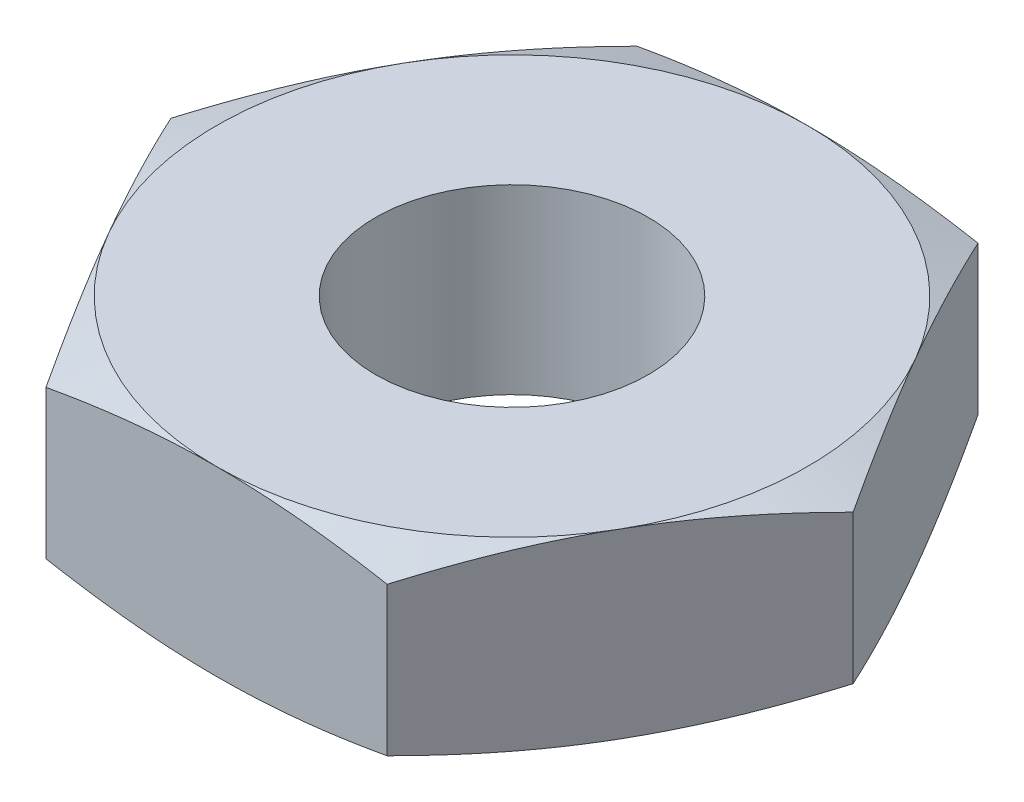
from build123d import *

# Parameters (mm, degrees)
HEX_PROFILE_SKETCH_R                  = 6
HEX_NUT_BODY_DEPTH                    = 4
CHAMFER_CIRCLE_SKETCH_OUTSIDE_W       = 163.26
CHAMFER_CIRCLE_SKETCH_OUTSIDE_H       = 159.238
CHAMFER_CIRCLE_SKETCH_OUTSIDE_R       = 13
TOP_CHAMFER_CUT_70DEG_DEPTH           = 22.408720964
TOP_CHAMFER_CUT_70DEG_DRAFT           = -70
BOTTOM_CHAMFER_MIRROR_COPY_1_SKETCH_W = 163.26
BOTTOM_CHAMFER_MIRROR_COPY_1_SKETCH_H = 159.238
BOTTOM_CHAMFER_MIRROR_COPY_1_SKETCH_R = 13
BOTTOM_CHAMFER_MIRROR_COPY_1_DEPTH    = 22.408720964
BOTTOM_CHAMFER_MIRROR_COPY_1_DRAFT    = -70


with BuildPart() as part:
    # Hex Profile Sketch → Hex Nut Body (new, symmetric)
    with BuildSketch(Plane(origin=(0, 0, 0), x_dir=(1, 0, 0), z_dir=(0, 1, 0))):
        Polygon((15.011106999, 0), (7.505553499, 13), (-7.505553499, 13), (-15.011106999, 0), (-7.505553499, -13), (7.505553499, -13), align=None)
        with Locations(Location((0, 0, 0), (0, 0, 270))):
            Circle(HEX_PROFILE_SKETCH_R, mode=Mode.SUBTRACT)
    extrude(amount=HEX_NUT_BODY_DEPTH, both=True)


with BuildPart() as top_chamfer_cut_70deg_tool:
    # Chamfer Circle Sketch outside → Top Chamfer Cut 70deg (with draft: the straight prism first)
    with BuildSketch(Plane(origin=(0, 4, 0), x_dir=(1, 0, 0), z_dir=(0, 1, 0))):
        Rectangle(CHAMFER_CIRCLE_SKETCH_OUTSIDE_W, CHAMFER_CIRCLE_SKETCH_OUTSIDE_H)
        Circle(CHAMFER_CIRCLE_SKETCH_OUTSIDE_R, mode=Mode.SUBTRACT)
    extrude(amount=-TOP_CHAMFER_CUT_70DEG_DEPTH)
    # Top Chamfer Cut 70deg: the draft: its side faces are tilted about the plane it starts from
    top_chamfer_cut_70deg_sides = [top_chamfer_cut_70deg_tool.faces().sort_by_distance(p)[0] for p in [
        (0, -7.204360482, 79.619),
        (81.63, -7.204360482, 0),
        (0, -7.204360482, -79.619),
        (-81.63, -7.204360482, 0),
        (-13, -7.204360482, 0),
    ]]
    draft(top_chamfer_cut_70deg_sides, Plane(origin=(0, 4, 0), x_dir=(1, 0, 0), z_dir=(0, 1, 0)), TOP_CHAMFER_CUT_70DEG_DRAFT)


with BuildPart() as part_1:
    add(part.part)

    # Top Chamfer Cut 70deg: cut by top_chamfer_cut_70deg_tool
    add(top_chamfer_cut_70deg_tool.part, mode=Mode.SUBTRACT)


with BuildPart() as bottom_chamfer_mirror_copy_1_tool:
    # Bottom Chamfer Mirror copy 1 sketch → Bottom Chamfer Mirror copy 1 (with draft: the straight prism first)
    with BuildSketch(Plane.XZ.offset(4)):
        Rectangle(BOTTOM_CHAMFER_MIRROR_COPY_1_SKETCH_W, BOTTOM_CHAMFER_MIRROR_COPY_1_SKETCH_H)
        Circle(BOTTOM_CHAMFER_MIRROR_COPY_1_SKETCH_R, mode=Mode.SUBTRACT)
    extrude(amount=-BOTTOM_CHAMFER_MIRROR_COPY_1_DEPTH)
    # Bottom Chamfer Mirror copy 1: the draft: its side faces are tilted about the plane it starts from
    bottom_chamfer_mirror_copy_1_sides = [bottom_chamfer_mirror_copy_1_tool.faces().sort_by_distance(p)[0] for p in [
        (0, 7.204360482, 79.619),
        (81.63, 7.204360482, 0),
        (0, 7.204360482, -79.619),
        (-81.63, 7.204360482, 0),
        (-13, 7.204360482, 0),
    ]]
    draft(bottom_chamfer_mirror_copy_1_sides, Plane.XZ.offset(4), BOTTOM_CHAMFER_MIRROR_COPY_1_DRAFT)


with BuildPart() as part_2:
    add(part_1.part)

    # Bottom Chamfer Mirror copy 1: cut by bottom_chamfer_mirror_copy_1_tool
    add(bottom_chamfer_mirror_copy_1_tool.part, mode=Mode.SUBTRACT)


solid = part_2.part
